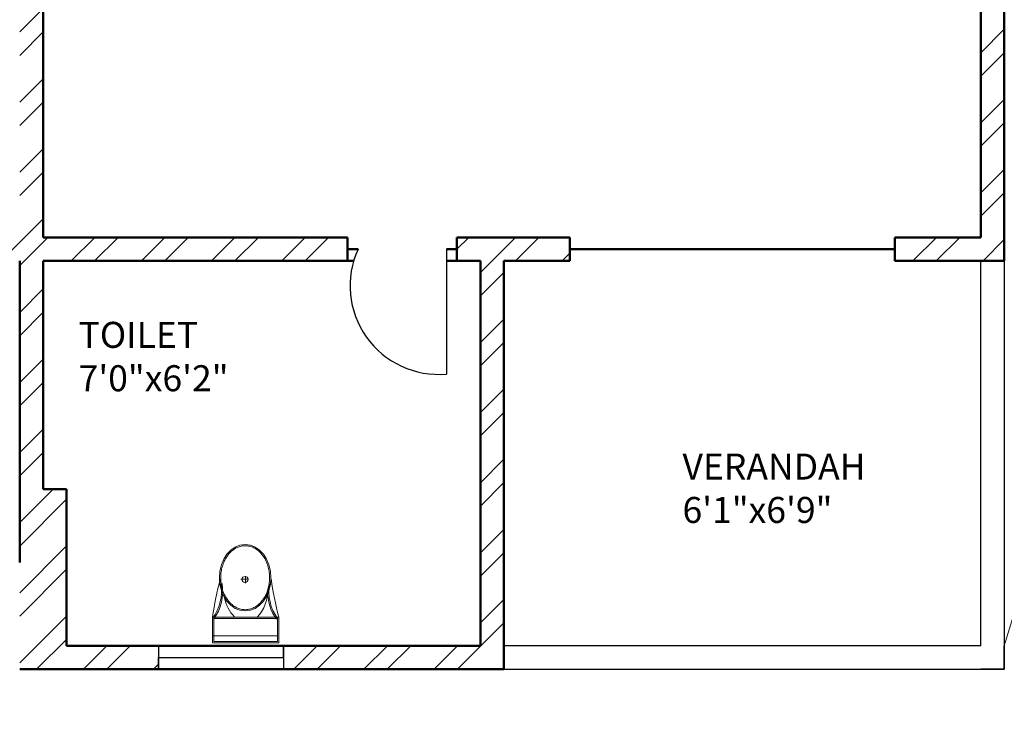
# Model space of a CAD drawing. Units: inches. Extents: x 1901 to 2863, y 888 to 2433.
# Tile 9 of 91: x 2154 to 2343, y 1216 to 1348. Entities that reach past the tile are written whole.
import ezdxf

# ---------------------------------------------------------------- set-up
doc = ezdxf.new("R2010")
doc.units = ezdxf.units.IN
for name, color, linetype, lineweight in [('A-ANNO-SYMB', 8, 'Continuous', 13), ('A-AREA-IDEN', 7, 'Continuous', 18), ('A-DOOR', 4, 'Continuous', 25), ('A-FLOR-FIXT', 9, 'Continuous', 18), ('A-FLOR-HRAL', 41, 'Continuous', 25), ('A-GLAZ', 3, 'Continuous', 25), ('A-WALL', 7, 'Continuous', 50), ('A-WALL-PATT', 8, 'Continuous', 13)]:
    doc.layers.add(name, color=color, linetype=linetype, lineweight=lineweight)
doc.styles.get("Standard").update_dxf_attribs({"font": 'arial.ttf'})

# ---------------------------------------------------------------- blocks, each defined once
blk = doc.blocks.new('A$C31115884')
for p, q in [((283.1, 497.7), (223.4, 497.7)), ((257.5, 466.4), (257.5, 523.2)), ((0, 200), (0, 0)), ((520, 200), (0, 200)), ((10, 190), (10, 10)), ((510, 190), (10, 190)), ((510, 10), (510, 190)), ((520, 0), (520, 200)), ((510, 54.5), (0, 54.5)), ((10, 10), (510, 10)), ((0, 0), (520, 0))]:
    blk.add_line(p, q)
blk.add_circle((255.6, 496.4), 23.6)
for centre, radius, start, end in [((2777.7, -204.6), 2807, 165.4549, 171.71327), ((-294.5, 403.3), 374.7, 324.20913, 9.34987), ((3237, 905), 2807, 188.28673, 194.5451), ((-294.5, 403.3), 364.7, 324.20913, 9.34987), ((139.5, 406.2), 293.5, 315.84364, 2.65635), ((805.8, 403.3), 374.7, 179.20365, 215.79087), ((805.8, 403.3), 364.7, 170.65013, 215.79087), ((383.6, 406.2), 293.5, 190.27735, 224.15636)]:
    blk.add_arc(centre, radius, start, end)
blk.add_ellipse((256.2, 509.9), major_axis=(0, -260.7), ratio=0.772727)
blk.add_open_spline([(256.2, 259.2), (263.1, 259.2), (270, 259.7), (287.8, 262.3), (298.7, 265.1), (319.9, 273.1), (330.2, 278.4), (350.1, 291.1), (359.7, 298.7), (377.7, 315.9), (386.2, 325.5), (401.7, 346.6), (408.8, 358.1), (421.3, 382.5), (426.8, 395.5), (435.9, 422.4), (439.5, 436.4), (444.8, 465.1), (446.5, 479.7), (447.9, 509.2), (447.6, 524), (445, 553.3), (442.7, 567.8), (436.3, 596), (432.1, 609.7), (421.9, 636), (416, 648.6), (402.5, 672.1), (395, 683), (378.6, 703), (369.8, 712.1), (351.1, 728), (341.3, 734.8), (320.9, 746.2), (310.4, 750.7), (288.9, 757.3), (278, 759.4), (256, 761), (245, 760.6), (223.1, 757.2), (212.3, 754.3), (191.1, 746.1), (180.8, 740.7), (160.9, 727.8), (151.4, 720.1), (133.5, 702.7), (125.1, 693), (109.6, 671.7), (102.6, 660.2), (90.2, 635.7), (84.9, 622.7), (76, 595.6), (72.4, 581.6), (67.2, 552.9), (65.6, 538.2), (64.4, 508.8), (64.8, 494), (67.5, 464.7), (69.9, 450.2), (76.6, 422), (80.8, 408.3), (91.1, 382.2), (97.2, 369.7), (110.8, 346.3), (118.4, 335.4), (134.8, 315.6), (143.7, 306.7), (162.4, 290.9), (172.3, 284.2), (192.8, 273), (203.3, 268.6), (224.8, 262.2), (235.8, 260.2), (249.9, 259.3), (253, 259.2), (256.2, 259.2)], degree=3, knots=[0, 0, 0, 0, 0.110105, 0.110105, 0.285049, 0.285049, 0.459994, 0.459994, 0.634938, 0.634938, 0.809882, 0.809882, 0.984827, 0.984827, 1.159771, 1.159771, 1.334715, 1.334715, 1.50966, 1.50966, 1.684604, 1.684604, 1.859549, 1.859549, 2.034493, 2.034493, 2.209437, 2.209437, 2.384382, 2.384382, 2.559326, 2.559326, 2.73427, 2.73427, 2.909215, 2.909215, 3.084159, 3.084159, 3.259103, 3.259103, 3.434048, 3.434048, 3.608992, 3.608992, 3.783936, 3.783936, 3.958881, 3.958881, 4.133825, 4.133825, 4.30877, 4.30877, 4.483714, 4.483714, 4.658658, 4.658658, 4.833603, 4.833603, 5.008547, 5.008547, 5.183491, 5.183491, 5.358436, 5.358436, 5.53338, 5.53338, 5.708324, 5.708324, 5.883269, 5.883269, 6.058213, 6.058213, 6.233158, 6.233158, 6.283185, 6.283185, 6.283185, 6.283185])
blk = doc.blocks.new('WIN-24')
for p, q in [((0, 4.5), (0, 0)), ((24, 2.25), (24, 4.5)), ((24, 4.5), (24, 0)), ((0, 0), (0, 2.25)), ((0, 2.25), (24, 2.25))]:
    blk.add_line(p, q)

msp = doc.modelspace()

# ---------------------------------------------------------------- hatches: boundary and pattern name
at = {"layer": 'A-WALL-PATT'}
h = msp.add_hatch(dxfattribs=at)
h.set_pattern_fill('ANSI32', color=256)
h.paths.add_polyline_path([(2192.5, 2274.13), (2141.26, 2274.13), (2141.26, 2269.63), (2192.5, 2269.63)])
h.paths.add_polyline_path([(2259.93, 2274.13), (2216.5, 2274.13), (2216.5, 2269.63), (2255.43, 2269.63), (2255.43, 2214.63), (2250.81, 2214.63), (2250.81, 2210.13), (2259.93, 2210.13), (2259.93, 2215.13), (2271.76, 2215.13), (2271.76, 2217.38), (2271.76, 2219.63), (2259.93, 2219.63)])
h.paths.add_polyline_path([(2171.43, 2269.63), (2166.93, 2269.63), (2166.93, 2219.63), (2121.24, 2219.63), (2121.24, 2215.13), (2166.93, 2215.13), (2166.93, 2083.13), (2161.81, 2083.13), (2161.81, 2078.63), (2171.43, 2078.63), (2177, 2078.63), (2177, 2080.88), (2177, 2083.13), (2171.43, 2083.13), (2171.43, 2210.13), (2230.91, 2210.13), (2230.91, 2212.38), (2230.91, 2214.63), (2171.43, 2214.63)])
h.paths.add_polyline_path([(2117.26, 2274.13), (2089.43, 2274.13), (2089.43, 2219.63), (2081.14, 2219.63), (2081.14, 2215.13), (2089.43, 2215.13), (2098, 2215.13), (2098, 2217.38), (2098, 2219.63), (2093.93, 2219.63), (2093.93, 2269.63), (2117.26, 2269.63), (2117.26, 2271.88)])
h.paths.add_polyline_path([(2343.43, 2219.63), (2329.29, 2219.63), (2329.29, 2215.13), (2338.93, 2215.13), (2338.93, 2184.74), (2343.43, 2184.74)])
h.paths.add_polyline_path([(2338.93, 2083.13), (2329.29, 2083.13), (2208.97, 2083.13), (2208.97, 2078.63), (2338.93, 2078.63)])
h.paths.add_polyline_path([(2343.43, 2136.74), (2338.93, 2136.74), (2338.93, 1872.63), (2343.43, 1872.63)])
h.paths.add_polyline_path([(2343.43, 1863.63), (2397.68, 1863.63), (2397.68, 1821.63), (2384.14, 1821.63), (2384.14, 1812.63), (2418.33, 1812.63), (2418.33, 1817.13), (2418.33, 1821.63), (2406.68, 1821.63), (2406.68, 1863.63), (2459.5, 1863.63), (2459.5, 1821.63), (2447.14, 1821.63), (2447.14, 1812.63), (2459.5, 1812.63), (2468.5, 1812.63), (2468.5, 1872.63), (2394.43, 1872.63), (2334.43, 1872.63), (2334.43, 1812.63), (2343.43, 1812.63), (2353.25, 1812.63), (2353.25, 1821.63), (2343.43, 1821.63)])
h.paths.add_polyline_path([(2510.01, 1872.63), (2468.5, 1872.63), (2468.5, 1868.13), (2510.01, 1868.13)])
h.paths.add_polyline_path([(2514.01, 1817.13), (2468.5, 1817.13), (2468.5, 1812.63), (2482.11, 1812.63), (2482.11, 1800.61), (2486.61, 1800.61), (2486.61, 1812.63), (2514.01, 1812.63)])
h.paths.add_polyline_path([(2299.25, 1814.88), (2299.25, 1817.13), (2295.93, 1817.13), (2295.93, 1854.17), (2293.68, 1854.17), (2291.43, 1854.17), (2291.43, 1817.13), (2266.11, 1817.13), (2266.11, 1812.63), (2299.25, 1812.63)])
h.paths.add_polyline_path([(2218.11, 1817.13), (2206.46, 1817.13), (2171.43, 1817.13), (2171.43, 1949.13), (2190.1, 1949.13), (2190.1, 1953.63), (2163.47, 1953.63), (2163.47, 1949.13), (2166.93, 1949.13), (2166.93, 1817.13), (2114.3, 1817.13), (2114.3, 1812.63), (2218.11, 1812.63)])
h.paths.add_polyline_path([(2029.43, 1970.92), (2024.93, 1970.92), (2024.93, 1912.72), (2029.43, 1912.72)])
h.paths.add_polyline_path([(2132.3, 1953.63), (2113.93, 1953.63), (2113.93, 1975.89), (2111.68, 1975.89), (2109.43, 1975.89), (2109.43, 1953.63), (2029.43, 1953.63), (2029.43, 1949.13), (2132.3, 1949.13)])
h.paths.add_polyline_path([(2029.43, 1853.61), (2029.31, 1853.61), (2029.31, 1853.61), (2029.43, 1853.61), (2029.43, 1864.72), (2024.93, 1864.72), (2024.93, 1812.63), (2066.3, 1812.63), (2066.3, 1814.88), (2066.3, 1817.13), (2029.43, 1817.13)])
h.paths.add_polyline_path([(2122.93, 2010.09), (2120.68, 2010.09), (2118.43, 2010.09), (2118.43, 2006.13), (2029.43, 2006.13), (2029.43, 2001.63), (2109.43, 2001.63), (2109.43, 1998.04), (2113.93, 1998.04), (2113.93, 2001.63), (2122.93, 2001.63)])
h.paths.add_polyline_path([(2029.43, 2031.38), (2024.93, 2031.38), (2024.93, 1994.92), (2027.18, 1994.92), (2029.43, 1994.92)])
h.paths.add_polyline_path([(2029.43, 2136.74), (2024.93, 2136.74), (2024.93, 2067.38), (2027.18, 2067.38), (2029.43, 2067.38)])
h.paths.add_polyline_path([(2125.62, 2083.13), (2029.43, 2083.13), (2029.43, 2078.63), (2118.43, 2078.63), (2118.43, 2030.71), (2122.93, 2030.71), (2122.93, 2078.63), (2125.62, 2078.63)])
h.paths.add_polyline_path([(2029.43, 2215.13), (2040.47, 2215.13), (2040.47, 2217.38), (2040.47, 2219.63), (2024.93, 2219.63), (2024.93, 2184.74), (2029.43, 2184.74), (2029.43, 2187.78)])
h.paths.add_polyline_path([(2686.43, 2274.13), (2659.28, 2274.13), (2659.28, 2269.63), (2681.93, 2269.63), (2681.93, 2219.63), (2676.82, 2219.63), (2676.82, 2215.13), (2681.93, 2215.13), (2697.01, 2215.13), (2697.01, 2217.38), (2697.01, 2219.63), (2686.43, 2219.63)])
h.paths.add_polyline_path([(2609.93, 2269.63), (2635.28, 2269.63), (2635.28, 2274.13), (2571.43, 2274.13), (2571.43, 2269.63), (2605.43, 2269.63), (2605.43, 2214.63), (2549.1, 2214.63), (2549.1, 2210.13), (2605.43, 2210.13), (2605.43, 2083.13), (2601.01, 2083.13), (2601.01, 2080.88), (2601.01, 2078.63), (2609.93, 2078.63), (2616.16, 2078.63), (2616.16, 2080.88), (2616.16, 2083.13), (2609.93, 2083.13), (2609.93, 2215.13), (2651.46, 2215.13), (2651.46, 2217.38), (2651.46, 2219.63), (2609.93, 2219.63)])
h.paths.add_polyline_path([(2521.43, 2269.63), (2547.43, 2269.63), (2547.43, 2271.88), (2547.43, 2274.13), (2516.93, 2274.13), (2516.93, 2219.63), (2506.41, 2219.63), (2506.41, 2215.13), (2516.93, 2215.13), (2516.93, 2210.13), (2525.4, 2210.13), (2525.4, 2212.38), (2525.4, 2214.63), (2521.43, 2214.63)])
h.paths.add_polyline_path([(2456.01, 2219.63), (2439.43, 2219.63), (2439.43, 2187.89), (2443.93, 2187.89), (2443.93, 2215.13), (2456.01, 2215.13)])
h.paths.add_polyline_path([(2752.93, 2219.63), (2739.48, 2219.63), (2739.48, 2215.13), (2748.43, 2215.13), (2748.43, 2187.89), (2752.93, 2187.89)])
h.paths.add_polyline_path([(2752.93, 2139.89), (2748.43, 2139.89), (2748.43, 2083.13), (2648.42, 2083.13), (2648.42, 2078.63), (2654.93, 2078.63), (2654.93, 2039.44), (2659.43, 2039.44), (2659.43, 2078.63), (2748.43, 2078.63), (2748.43, 2063.43), (2752.93, 2063.43)])
h.paths.add_polyline_path([(2752.93, 2010.63), (2659.43, 2010.63), (2659.43, 2015.65), (2654.93, 2015.65), (2654.93, 2010.63), (2605.43, 2010.63), (2605.43, 1920.97), (2609.93, 1920.97), (2609.93, 2006.13), (2748.43, 2006.13), (2748.43, 1982.47), (2752.93, 1982.47)])
h.paths.add_polyline_path([(2752.93, 2027.43), (2748.43, 2027.43), (2748.43, 2010.63), (2752.93, 2010.63)])
h.paths.add_polyline_path([(2748.43, 1886.13), (2609.93, 1886.13), (2609.93, 1889.72), (2605.43, 1889.72), (2605.43, 1861.26), (2609.93, 1861.26), (2609.93, 1881.63), (2748.43, 1881.63)])
h.paths.add_polyline_path([(2456.86, 2228.83), (2498.4, 2228.83), (2498.4, 2247.49), (2456.86, 2247.49)], flags=9)
h.paths.add_polyline_path([(2038.6, 2237.42), (2080.17, 2237.42), (2080.17, 2256.08), (2038.6, 2256.08)], flags=9)
h.paths.add_polyline_path([(2292.01, 1062.39), (2539.93, 1062.39), (2539.93, 1099.49), (2292.01, 1099.49)], flags=9)
h.paths.add_polyline_path([(2424.91, 1832.25), (2448.51, 1832.25), (2448.51, 1846.68), (2424.91, 1846.68)], flags=25)
h.paths.add_polyline_path([(2359.08, 1832.25), (2382.68, 1832.25), (2382.68, 1846.68), (2359.08, 1846.68)], flags=25)
h.paths.add_polyline_path([(2352.9, 1684.8), (2367.54, 1684.8), (2367.54, 1697.17), (2352.9, 1697.17)], flags=9)
h.paths.add_polyline_path([(2079.29, 1755.83), (2169.02, 1755.83), (2169.02, 1774.37), (2079.29, 1774.37)], flags=9)
h.paths.add_polyline_path([(2404.09, 1373.86), (2404.09, 1463.59), (2385.54, 1463.59), (2385.54, 1373.86)], flags=9)
h.paths.add_polyline_path([(2268.09, 2236.37), (2309.64, 2236.37), (2309.64, 2255.03), (2268.09, 2255.03)], flags=9)
h.paths.add_polyline_path([(2575.96, 1700.95), (2665.7, 1700.95), (2665.7, 1719.5), (2575.96, 1719.5)], flags=9)
h.paths.add_polyline_path([(2302.96, 1878.47), (2329.52, 1878.47), (2329.52, 1888.78), (2302.96, 1888.78)], flags=9)
h.paths.add_polyline_path([(2097.42, 2240.58), (2126.57, 2240.58), (2126.57, 2259.23), (2097.42, 2259.23)], flags=9)
h.paths.add_polyline_path([(2208.72, 2246.12), (2237.88, 2246.12), (2237.88, 2264.78), (2208.72, 2264.78)], flags=9)
h.paths.add_polyline_path([(2038.15, 1925.96), (2076.99, 1925.96), (2076.99, 1944.62), (2038.15, 1944.62)], flags=9)
h.paths.add_polyline_path([(2239.14, 1926.67), (2288.46, 1926.67), (2288.46, 1945.33), (2239.14, 1945.33)], flags=9)
h.paths.add_polyline_path([(2175.43, 2007.33), (2212.36, 2007.33), (2212.36, 2025.99), (2175.43, 2025.99)], flags=9)
h.paths.add_polyline_path([(2225.03, 2091.79), (2263.87, 2091.79), (2263.87, 2110.45), (2225.03, 2110.45)], flags=9)
h.paths.add_polyline_path([(2035.4, 2098.48), (2074.24, 2098.48), (2074.24, 2117.14), (2035.4, 2117.14)], flags=9)
h.paths.add_polyline_path([(2050.1, 2029.21), (2083.26, 2029.21), (2083.26, 2047.87), (2050.1, 2047.87)], flags=9)
h.paths.add_polyline_path([(2069.68, 1956.72), (2098.83, 1956.72), (2098.83, 1975.38), (2069.68, 1975.38)], flags=25)
h.paths.add_polyline_path([(2328.62, 1753.34), (2361.66, 1753.34), (2361.66, 1771.99), (2328.62, 1771.99)], flags=9)
h.paths.add_polyline_path([(2395.16, 2060.89), (2395.16, 2140.65), (2378.68, 2140.65), (2378.68, 2060.89)], flags=9)
h.paths.add_polyline_path([(2463.73, 2059.02), (2492.89, 2059.02), (2492.89, 2077.68), (2463.73, 2077.68)], flags=9)
h.paths.add_polyline_path([(2458.03, 2181.54), (2496.87, 2181.54), (2496.87, 2200.19), (2458.03, 2200.19)], flags=9)
h.paths.add_polyline_path([(2527.58, 2243.07), (2556.73, 2243.07), (2556.73, 2261.73), (2527.58, 2261.73)], flags=9)
h.paths.add_polyline_path([(2694.46, 2232.77), (2736.03, 2232.77), (2736.03, 2251.42), (2694.46, 2251.42)], flags=9)
h.paths.add_polyline_path([(2637.82, 2249.22), (2666.98, 2249.22), (2666.98, 2267.88), (2637.82, 2267.88)], flags=9)
h.paths.add_polyline_path([(2623.69, 2183.54), (2662.53, 2183.54), (2662.53, 2202.2), (2623.69, 2202.2)], flags=9)
h.paths.add_polyline_path([(2691.97, 2021.5), (2725.12, 2021.5), (2725.12, 2040.16), (2691.97, 2040.16)], flags=9)
h.paths.add_polyline_path([(2621.04, 1975.91), (2662.34, 1975.91), (2662.34, 1994.57), (2621.04, 1994.57)], flags=25)
h.paths.add_polyline_path([(2479.03, 1927.62), (2519.84, 1927.62), (2519.84, 1946.28), (2479.03, 1946.28)], flags=9)
h.paths.add_polyline_path([(2670.94, 1849.08), (2716.01, 1849.08), (2716.01, 1867.73), (2670.94, 1867.73)], flags=9)
h.paths.add_polyline_path([(2523.61, 1782.96), (2550.17, 1782.96), (2550.17, 1793.26), (2523.61, 1793.26)], flags=9)
h.paths.add_polyline_path([(2450.84, 1207.33), (2492.39, 1207.33), (2492.39, 1225.99), (2450.84, 1225.99)], flags=9)
h.paths.add_polyline_path([(2527.75, 1203.84), (2556.91, 1203.84), (2556.91, 1222.5), (2527.75, 1222.5)], flags=9)
h.paths.add_polyline_path([(2639.11, 1207.2), (2668.27, 1207.2), (2668.27, 1225.86), (2639.11, 1225.86)], flags=9)
h.paths.add_polyline_path([(2692.59, 1218.97), (2734.17, 1218.97), (2734.17, 1237.62), (2692.59, 1237.62)], flags=9)
h.paths.add_polyline_path([(2669.27, 1366.33), (2708.11, 1366.33), (2708.11, 1384.99), (2669.27, 1384.99)], flags=9)
h.paths.add_polyline_path([(2463.31, 1358.03), (2502.15, 1358.03), (2502.15, 1376.69), (2463.31, 1376.69)], flags=9)
h.paths.add_polyline_path([(2494.72, 1449.96), (2531.65, 1449.96), (2531.65, 1468.62), (2494.72, 1468.62)], flags=9)
h.paths.add_polyline_path([(2675.57, 1422.16), (2708.72, 1422.16), (2708.72, 1440.81), (2675.57, 1440.81)], flags=9)
h.paths.add_polyline_path([(2685.63, 1493.89), (2714.79, 1493.89), (2714.79, 1512.55), (2685.63, 1512.55)], flags=9)
h.paths.add_polyline_path([(2686.8, 1529.91), (2725.65, 1529.91), (2725.65, 1548.57), (2686.8, 1548.57)], flags=9)
h.paths.add_polyline_path([(2503.65, 1537.99), (2552.97, 1537.99), (2552.97, 1556.65), (2503.65, 1556.65)], flags=9)
h.paths.add_polyline_path([(2291.71, 1643.5), (2318.28, 1643.5), (2318.28, 1653.81), (2291.71, 1653.81)], flags=9)
h.paths.add_polyline_path([(2450.63, 1610.52), (2477.19, 1610.52), (2477.19, 1620.82), (2450.63, 1620.82)], flags=9)
h.paths.add_polyline_path([(2359.99, 1551.81), (2422.25, 1551.81), (2422.25, 1562.12), (2359.99, 1562.12)], flags=9)
h.paths.add_polyline_path([(2280.11, 1249.01), (2321.65, 1249.01), (2321.65, 1267.66), (2280.11, 1267.66)], flags=9)
h.paths.add_polyline_path([(2164.06, 1274.23), (2193.22, 1274.23), (2193.22, 1292.89), (2164.06, 1292.89)], flags=9)
h.paths.add_polyline_path([(2118.21, 1277.69), (2151.25, 1277.69), (2151.25, 1296.35), (2118.21, 1296.35)], flags=9)
h.paths.add_polyline_path([(2031.95, 1268.53), (2073.52, 1268.53), (2073.52, 1287.19), (2031.95, 1287.19)], flags=9)
h.paths.add_polyline_path([(2050.2, 1409.08), (2089.04, 1409.08), (2089.04, 1427.74), (2050.2, 1427.74)], flags=9)
h.paths.add_polyline_path([(2243.74, 1421.03), (2282.58, 1421.03), (2282.58, 1439.69), (2243.74, 1439.69)], flags=9)
h.paths.add_polyline_path([(2190.75, 1509.77), (2231.56, 1509.77), (2231.56, 1528.43), (2190.75, 1528.43)], flags=9)
h.paths.add_polyline_path([(2058.39, 1475.42), (2091.55, 1475.42), (2091.55, 1494.07), (2058.39, 1494.07)], flags=9)
h.paths.add_polyline_path([(2062.45, 1553.09), (2091.6, 1553.09), (2091.6, 1571.75), (2062.45, 1571.75)], flags=9)
h.paths.add_polyline_path([(2219.52, 1590.37), (2266.15, 1590.37), (2266.15, 1609.02), (2219.52, 1609.02)], flags=9)
h.paths.add_polyline_path([(2041.07, 1584.19), (2079.91, 1584.19), (2079.91, 1602.85), (2041.07, 1602.85)], flags=9)
h = msp.add_hatch(dxfattribs=at)
h.set_pattern_fill('ANSI32', color=256)
h.paths.add_polyline_path([(2443.93, 2139.89), (2439.43, 2139.89), (2439.43, 2069.35), (2441.68, 2069.35), (2443.93, 2069.35), (2443.93, 2078.63), (2521.93, 2078.63), (2521.93, 2075.07), (2524.18, 2075.07), (2526.43, 2075.07), (2526.43, 2078.63), (2571.75, 2078.63), (2571.75, 2080.88), (2571.75, 2083.13), (2443.93, 2083.13)])
h.paths.add_polyline_path([(2526.43, 2054.63), (2524.18, 2054.63), (2521.93, 2054.63), (2521.93, 2030.63), (2443.93, 2030.63), (2443.93, 2045.35), (2439.43, 2045.35), (2439.43, 1983.87), (2443.93, 1983.87), (2443.93, 2026.13), (2521.93, 2026.13), (2526.43, 2026.13)])
h.paths.add_polyline_path([(2443.93, 1923.87), (2439.43, 1923.87), (2439.43, 1872.63), (2443.93, 1872.63)])
h.paths.add_polyline_path([(2636.23, 1766.13), (2609.93, 1766.13), (2609.93, 1779.79), (2605.43, 1779.79), (2605.43, 1766.13), (2486.61, 1766.13), (2486.61, 1770.67), (2482.11, 1770.67), (2482.11, 1766.13), (2482.11, 1761.63), (2636.23, 1761.63), (2636.23, 1763.88)])
h.paths.add_polyline_path([(2519.54, 1663.38), (2519.54, 1665.63), (2494.93, 1665.63), (2481.83, 1665.63), (2481.83, 1663.38), (2481.83, 1661.13), (2490.43, 1661.13), (2490.43, 1640.16), (2494.93, 1640.16), (2494.93, 1661.13), (2519.54, 1661.13)])
h.paths.add_polyline_path([(2443.93, 1712.13), (2443.93, 1716.63), (2414.46, 1716.63), (2414.46, 1712.13), (2439.43, 1712.13), (2439.43, 1545.51), (2443.93, 1545.51), (2443.93, 1661.13), (2448.47, 1661.13), (2448.47, 1665.63), (2443.93, 1665.63)])
h.paths.add_polyline_path([(2343.43, 1712.13), (2365.52, 1712.13), (2365.52, 1714.38), (2365.52, 1716.63), (2333.87, 1716.63), (2333.87, 1714.38), (2333.87, 1712.13), (2338.93, 1712.13), (2338.93, 1575.63), (2338.93, 1545.51), (2343.43, 1545.51), (2343.43, 1547.51), (2343.43, 1580.13)])
h.paths.add_polyline_path([(2752.93, 1665.63), (2579.54, 1665.63), (2579.54, 1661.13), (2615.93, 1661.13), (2615.93, 1529.13), (2598.93, 1529.13), (2598.93, 1524.63), (2623.13, 1524.63), (2623.13, 1526.88), (2623.13, 1529.13), (2620.43, 1529.13), (2620.43, 1661.13), (2748.43, 1661.13), (2748.43, 1633.5), (2752.93, 1633.5)])
h.paths.add_polyline_path([(2752.93, 1419.93), (2748.43, 1419.93), (2748.43, 1400.13), (2659.43, 1400.13), (2659.43, 1444.33), (2657.18, 1444.33), (2654.93, 1444.33), (2654.93, 1400.13), (2643.65, 1400.13), (2643.65, 1395.63), (2748.43, 1395.63), (2748.43, 1364.04), (2752.93, 1364.04)])
h.paths.add_polyline_path([(2752.93, 1492.88), (2748.43, 1492.88), (2748.43, 1476.63), (2667.43, 1476.63), (2667.43, 1479.71), (2665.18, 1479.71), (2662.93, 1479.71), (2662.93, 1476.63), (2654.93, 1476.63), (2654.93, 1469.54), (2659.43, 1469.54), (2659.43, 1472.13), (2748.43, 1472.13), (2748.43, 1455.93), (2752.93, 1455.93)])
h.paths.add_polyline_path([(2752.93, 1304.04), (2748.43, 1304.04), (2748.43, 1263.63), (2738.66, 1263.63), (2738.66, 1259.13), (2752.93, 1259.13)])
h.paths.add_polyline_path([(2685.93, 1259.13), (2695.49, 1259.13), (2695.49, 1261.38), (2695.49, 1263.63), (2677.84, 1263.63), (2677.84, 1261.38), (2677.84, 1259.13), (2681.43, 1259.13), (2681.43, 1203.63), (2653.28, 1203.63), (2653.28, 1199.13), (2685.93, 1199.13), (2685.93, 1203.63)])
h.paths.add_polyline_path([(2609.43, 1395.63), (2611.85, 1395.63), (2611.85, 1400.13), (2598.89, 1400.13), (2598.89, 1397.88), (2598.89, 1395.63), (2604.93, 1395.63), (2604.93, 1268.13), (2554.73, 1268.13), (2554.73, 1265.88), (2554.73, 1263.63), (2604.93, 1263.63), (2604.93, 1203.63), (2571.31, 1203.63), (2571.31, 1199.13), (2604.93, 1199.13), (2629.28, 1199.13), (2629.28, 1201.38), (2629.28, 1203.63), (2609.43, 1203.63), (2609.43, 1258.63), (2609.43, 1259.13), (2654.8, 1259.13), (2654.8, 1263.63), (2609.43, 1263.63)])
h.paths.add_polyline_path([(2443.93, 1304.04), (2439.43, 1304.04), (2439.43, 1259.13), (2443.93, 1259.13), (2456.16, 1259.13), (2456.16, 1261.38), (2456.16, 1263.63), (2443.93, 1263.63)])
h.paths.add_polyline_path([(2525.43, 1263.63), (2531.78, 1263.63), (2531.78, 1268.13), (2520.93, 1268.13), (2520.93, 1263.63), (2511.41, 1263.63), (2511.41, 1259.13), (2520.93, 1259.13), (2520.93, 1199.13), (2547.31, 1199.13), (2547.31, 1201.38), (2547.31, 1203.63), (2525.43, 1203.63)])
h.paths.add_polyline_path([(2443.93, 1434.84), (2439.43, 1434.84), (2439.43, 1364.04), (2441.68, 1364.04), (2443.93, 1364.04)])
h.paths.add_polyline_path([(2567.13, 1400.13), (2443.93, 1400.13), (2443.93, 1395.63), (2567.13, 1395.63)])
h.paths.add_polyline_path([(2443.93, 1545.51), (2439.43, 1545.51), (2439.43, 1494.84), (2443.93, 1494.84)])
h.paths.add_polyline_path([(2494.93, 1553.35), (2492.68, 1553.35), (2490.43, 1553.35), (2490.43, 1524.63), (2494.93, 1524.63), (2525.94, 1524.63), (2525.94, 1526.88), (2525.94, 1529.13), (2494.93, 1529.13)])
h.paths.add_polyline_path([(2752.93, 1573.5), (2748.43, 1573.5), (2748.43, 1529.13), (2657.76, 1529.13), (2657.76, 1524.63), (2662.93, 1524.63), (2662.93, 1498.63), (2667.43, 1498.63), (2667.43, 1524.63), (2748.43, 1524.63), (2748.43, 1516.88), (2752.93, 1516.88)])
h.paths.add_polyline_path([(2038.6, 2237.42), (2080.17, 2237.42), (2080.17, 2256.08), (2038.6, 2256.08)], flags=9)
h.paths.add_polyline_path([(2292.01, 1062.39), (2539.93, 1062.39), (2539.93, 1099.49), (2292.01, 1099.49)], flags=9)
h.paths.add_polyline_path([(2424.91, 1832.25), (2448.51, 1832.25), (2448.51, 1846.68), (2424.91, 1846.68)], flags=9)
h.paths.add_polyline_path([(2359.08, 1832.25), (2382.68, 1832.25), (2382.68, 1846.68), (2359.08, 1846.68)], flags=9)
h.paths.add_polyline_path([(2352.9, 1684.8), (2367.54, 1684.8), (2367.54, 1697.17), (2352.9, 1697.17)], flags=9)
h.paths.add_polyline_path([(2079.29, 1755.83), (2169.02, 1755.83), (2169.02, 1774.37), (2079.29, 1774.37)], flags=9)
h.paths.add_polyline_path([(2404.09, 1373.86), (2404.09, 1463.59), (2385.54, 1463.59), (2385.54, 1373.86)], flags=9)
h.paths.add_polyline_path([(2268.09, 2236.37), (2309.64, 2236.37), (2309.64, 2255.03), (2268.09, 2255.03)], flags=9)
h.paths.add_polyline_path([(2575.96, 1700.95), (2665.7, 1700.95), (2665.7, 1719.5), (2575.96, 1719.5)], flags=9)
h.paths.add_polyline_path([(2302.96, 1878.47), (2329.52, 1878.47), (2329.52, 1888.78), (2302.96, 1888.78)], flags=9)
h.paths.add_polyline_path([(2097.42, 2240.58), (2126.57, 2240.58), (2126.57, 2259.23), (2097.42, 2259.23)], flags=9)
h.paths.add_polyline_path([(2208.72, 2246.12), (2237.88, 2246.12), (2237.88, 2264.78), (2208.72, 2264.78)], flags=9)
h.paths.add_polyline_path([(2038.15, 1925.96), (2076.99, 1925.96), (2076.99, 1944.62), (2038.15, 1944.62)], flags=9)
h.paths.add_polyline_path([(2239.14, 1926.67), (2288.46, 1926.67), (2288.46, 1945.33), (2239.14, 1945.33)], flags=9)
h.paths.add_polyline_path([(2175.43, 2007.33), (2212.36, 2007.33), (2212.36, 2025.99), (2175.43, 2025.99)], flags=9)
h.paths.add_polyline_path([(2225.03, 2091.79), (2263.87, 2091.79), (2263.87, 2110.45), (2225.03, 2110.45)], flags=9)
h.paths.add_polyline_path([(2035.4, 2098.48), (2074.24, 2098.48), (2074.24, 2117.14), (2035.4, 2117.14)], flags=9)
h.paths.add_polyline_path([(2050.1, 2029.21), (2083.26, 2029.21), (2083.26, 2047.87), (2050.1, 2047.87)], flags=9)
h.paths.add_polyline_path([(2069.68, 1956.72), (2098.83, 1956.72), (2098.83, 1975.38), (2069.68, 1975.38)], flags=9)
h.paths.add_polyline_path([(2328.62, 1753.34), (2361.66, 1753.34), (2361.66, 1771.99), (2328.62, 1771.99)], flags=9)
h.paths.add_polyline_path([(2395.16, 2060.89), (2395.16, 2140.65), (2378.68, 2140.65), (2378.68, 2060.89)], flags=9)
h.paths.add_polyline_path([(2463.73, 2059.02), (2492.89, 2059.02), (2492.89, 2077.68), (2463.73, 2077.68)], flags=9)
h.paths.add_polyline_path([(2458.03, 2181.54), (2496.87, 2181.54), (2496.87, 2200.19), (2458.03, 2200.19)], flags=9)
h.paths.add_polyline_path([(2456.86, 2228.83), (2498.4, 2228.83), (2498.4, 2247.49), (2456.86, 2247.49)], flags=9)
h.paths.add_polyline_path([(2527.58, 2243.07), (2556.73, 2243.07), (2556.73, 2261.73), (2527.58, 2261.73)], flags=9)
h.paths.add_polyline_path([(2694.46, 2232.77), (2736.03, 2232.77), (2736.03, 2251.42), (2694.46, 2251.42)], flags=9)
h.paths.add_polyline_path([(2637.82, 2249.22), (2666.98, 2249.22), (2666.98, 2267.88), (2637.82, 2267.88)], flags=9)
h.paths.add_polyline_path([(2623.69, 2183.54), (2662.53, 2183.54), (2662.53, 2202.2), (2623.69, 2202.2)], flags=9)
h.paths.add_polyline_path([(2691.97, 2021.5), (2725.12, 2021.5), (2725.12, 2040.16), (2691.97, 2040.16)], flags=9)
h.paths.add_polyline_path([(2621.04, 1975.91), (2662.34, 1975.91), (2662.34, 1994.57), (2621.04, 1994.57)], flags=9)
h.paths.add_polyline_path([(2479.03, 1927.62), (2519.84, 1927.62), (2519.84, 1946.28), (2479.03, 1946.28)], flags=9)
h.paths.add_polyline_path([(2670.94, 1849.08), (2716.01, 1849.08), (2716.01, 1867.73), (2670.94, 1867.73)], flags=9)
h.paths.add_polyline_path([(2523.61, 1782.96), (2550.17, 1782.96), (2550.17, 1793.26), (2523.61, 1793.26)], flags=9)
h.paths.add_polyline_path([(2450.84, 1207.33), (2492.39, 1207.33), (2492.39, 1225.99), (2450.84, 1225.99)], flags=9)
h.paths.add_polyline_path([(2527.75, 1203.84), (2556.91, 1203.84), (2556.91, 1222.5), (2527.75, 1222.5)], flags=9)
h.paths.add_polyline_path([(2639.11, 1207.2), (2668.27, 1207.2), (2668.27, 1225.86), (2639.11, 1225.86)], flags=9)
h.paths.add_polyline_path([(2692.59, 1218.97), (2734.17, 1218.97), (2734.17, 1237.62), (2692.59, 1237.62)], flags=9)
h.paths.add_polyline_path([(2669.27, 1366.33), (2708.11, 1366.33), (2708.11, 1384.99), (2669.27, 1384.99)], flags=25)
h.paths.add_polyline_path([(2463.31, 1358.03), (2502.15, 1358.03), (2502.15, 1376.69), (2463.31, 1376.69)], flags=9)
h.paths.add_polyline_path([(2494.72, 1449.96), (2531.65, 1449.96), (2531.65, 1468.62), (2494.72, 1468.62)], flags=9)
h.paths.add_polyline_path([(2675.57, 1422.16), (2708.72, 1422.16), (2708.72, 1440.81), (2675.57, 1440.81)], flags=25)
h.paths.add_polyline_path([(2685.63, 1493.89), (2714.79, 1493.89), (2714.79, 1512.55), (2685.63, 1512.55)], flags=9)
h.paths.add_polyline_path([(2686.8, 1529.91), (2725.65, 1529.91), (2725.65, 1548.57), (2686.8, 1548.57)], flags=25)
h.paths.add_polyline_path([(2503.65, 1537.99), (2552.97, 1537.99), (2552.97, 1556.65), (2503.65, 1556.65)], flags=9)
h.paths.add_polyline_path([(2291.71, 1643.5), (2318.28, 1643.5), (2318.28, 1653.81), (2291.71, 1653.81)], flags=9)
h.paths.add_polyline_path([(2450.63, 1610.52), (2477.19, 1610.52), (2477.19, 1620.82), (2450.63, 1620.82)], flags=9)
h.paths.add_polyline_path([(2359.99, 1551.81), (2422.25, 1551.81), (2422.25, 1562.12), (2359.99, 1562.12)], flags=9)
h.paths.add_polyline_path([(2280.11, 1249.01), (2321.65, 1249.01), (2321.65, 1267.66), (2280.11, 1267.66)], flags=9)
h.paths.add_polyline_path([(2164.06, 1274.23), (2193.22, 1274.23), (2193.22, 1292.89), (2164.06, 1292.89)], flags=9)
h.paths.add_polyline_path([(2118.21, 1277.69), (2151.25, 1277.69), (2151.25, 1296.35), (2118.21, 1296.35)], flags=9)
h.paths.add_polyline_path([(2031.95, 1268.53), (2073.52, 1268.53), (2073.52, 1287.19), (2031.95, 1287.19)], flags=9)
h.paths.add_polyline_path([(2050.2, 1409.08), (2089.04, 1409.08), (2089.04, 1427.74), (2050.2, 1427.74)], flags=9)
h.paths.add_polyline_path([(2243.74, 1421.03), (2282.58, 1421.03), (2282.58, 1439.69), (2243.74, 1439.69)], flags=9)
h.paths.add_polyline_path([(2190.75, 1509.77), (2231.56, 1509.77), (2231.56, 1528.43), (2190.75, 1528.43)], flags=9)
h.paths.add_polyline_path([(2058.39, 1475.42), (2091.55, 1475.42), (2091.55, 1494.07), (2058.39, 1494.07)], flags=9)
h.paths.add_polyline_path([(2062.45, 1553.09), (2091.6, 1553.09), (2091.6, 1571.75), (2062.45, 1571.75)], flags=9)
h.paths.add_polyline_path([(2219.52, 1590.37), (2266.15, 1590.37), (2266.15, 1609.02), (2219.52, 1609.02)], flags=9)
h.paths.add_polyline_path([(2041.07, 1584.19), (2079.91, 1584.19), (2079.91, 1602.85), (2041.07, 1602.85)], flags=9)
h = msp.add_hatch(dxfattribs=at)
h.set_pattern_fill('ANSI32', color=256)
h.paths.add_polyline_path([(2182.93, 1716.63), (2024.93, 1716.63), (2024.93, 1681.7), (2029.33, 1681.7), (2029.33, 1712.13), (2154.33, 1712.13), (2154.33, 1580.13), (2148.52, 1580.13), (2148.52, 1577.88), (2148.52, 1575.63), (2194.93, 1575.63), (2194.93, 1580.13), (2158.83, 1580.13), (2158.83, 1712.13), (2182.93, 1712.13)])
h.paths.add_polyline_path([(2301.07, 1716.63), (2242.93, 1716.63), (2242.93, 1712.13), (2283.83, 1712.13), (2283.83, 1685.54), (2288.33, 1685.54), (2288.33, 1712.13), (2301.07, 1712.13)])
h.paths.add_polyline_path([(2288.33, 1600.41), (2286.08, 1600.41), (2283.83, 1600.41), (2283.83, 1580.13), (2270.6, 1580.13), (2270.6, 1575.63), (2288.33, 1575.63)])
h.paths.add_polyline_path([(2295.93, 1953.63), (2271.45, 1953.63), (2271.45, 1949.13), (2291.43, 1949.13), (2291.43, 1941.24), (2295.93, 1941.24)])
h.paths.add_polyline_path([(2098.38, 1244.13), (2082.33, 1244.13), (2082.33, 1302.13), (2086.52, 1302.13), (2086.52, 1306.63), (2067.46, 1306.63), (2067.46, 1302.13), (2077.83, 1302.13), (2077.83, 1239.63), (2098.38, 1239.63), (2098.38, 1241.88)])
h.paths.add_polyline_path([(2217.31, 1306.63), (2158.83, 1306.63), (2158.83, 1451.63), (2162.72, 1451.63), (2162.72, 1453.88), (2162.72, 1456.13), (2154.33, 1456.13), (2154.33, 1443.13), (2151.91, 1443.13), (2151.91, 1438.63), (2154.33, 1438.63), (2154.33, 1306.63), (2109.31, 1306.63), (2109.31, 1304.38), (2109.31, 1302.13), (2154.33, 1302.13), (2154.33, 1244.13), (2122.38, 1244.13), (2122.38, 1239.63), (2154.33, 1239.63), (2154.33, 1223.63), (2163.33, 1223.63), (2181.01, 1223.63), (2181.01, 1225.88), (2181.01, 1228.13), (2163.33, 1228.13), (2163.33, 1258.22), (2158.83, 1258.22), (2158.83, 1302.13), (2217.31, 1302.13)])
h.paths.add_polyline_path([(2259.99, 1306.63), (2238.3, 1306.63), (2238.3, 1304.38), (2238.3, 1302.13), (2242.83, 1302.13), (2242.83, 1228.13), (2205.01, 1228.13), (2205.01, 1223.63), (2247.33, 1223.63), (2247.33, 1302.13), (2259.99, 1302.13), (2259.99, 1304.38)])
h.paths.add_polyline_path([(2343.43, 1361.7), (2338.93, 1361.7), (2338.93, 1306.63), (2322.38, 1306.63), (2322.38, 1302.13), (2343.43, 1302.13)])
h.paths.add_polyline_path([(2343.43, 1470.4), (2338.93, 1470.4), (2338.93, 1456.13), (2193.73, 1456.13), (2193.73, 1453.88), (2193.73, 1451.63), (2338.93, 1451.63), (2338.93, 1421.7), (2343.43, 1421.7)])
h.paths.add_polyline_path([(2343.43, 1545.51), (2338.93, 1545.51), (2338.93, 1530.4), (2343.43, 1530.4)])
h.paths.add_polyline_path([(2029.33, 1466.83), (2024.93, 1466.83), (2024.93, 1409.82), (2029.33, 1409.82)])
h.paths.add_polyline_path([(2122.84, 1440.88), (2122.84, 1443.13), (2121.83, 1443.13), (2121.83, 1498.18), (2119.58, 1498.18), (2117.33, 1498.18), (2117.33, 1443.13), (2029.33, 1443.13), (2029.33, 1438.63), (2122.84, 1438.63)])
h.paths.add_polyline_path([(2029.33, 1543.05), (2024.93, 1543.05), (2024.93, 1502.83), (2029.33, 1502.83)])
h.paths.add_polyline_path([(2029.33, 1621.7), (2024.93, 1621.7), (2024.93, 1567.05), (2027.13, 1567.05), (2029.33, 1567.05), (2029.33, 1575.63), (2109.33, 1575.63), (2109.33, 1554.71), (2113.83, 1554.71), (2113.83, 1575.63), (2115.8, 1575.63), (2115.8, 1577.88), (2115.8, 1580.13), (2029.33, 1580.13)])
h.paths.add_polyline_path([(2121.83, 1527.63), (2117.33, 1527.63), (2113.83, 1527.63), (2113.83, 1533.01), (2111.58, 1533.01), (2109.33, 1533.01), (2109.33, 1527.63), (2029.33, 1527.63), (2029.33, 1523.13), (2117.33, 1523.13), (2117.33, 1519.43), (2121.83, 1519.43)])
h.paths.add_polyline_path([(2029.33, 1349.82), (2024.93, 1349.82), (2024.93, 1302.13), (2036.28, 1302.13), (2036.28, 1306.63), (2029.33, 1306.63)])

# ---------------------------------------------------------------- linework, layer by layer
at = {"layer": 'A-ANNO-SYMB'}
msp.add_line((2343.43, 1228.13), (2439.43, 1545.51), dxfattribs=at)
at = {"layer": 'A-DOOR'}
msp.add_line((2236.3, 1304.38), (2236.3, 1280.38), dxfattribs=at)
msp.add_arc((2234.79, 1297.33), 17.02, 155.518, 275.0742, dxfattribs=at)
at = {"layer": 'A-FLOR-HRAL'}
for p, q in [((2338.93, 1228.13), (2338.93, 1302.13)), ((2343.43, 1302.13), (2343.43, 1223.63)), ((2338.93, 1228.13), (2247.33, 1228.13)), ((2343.43, 1223.63), (2343.43, 1228.13)), ((2247.33, 1223.63), (2343.43, 1223.63)), ((2343.43, 1223.63), (2338.93, 1223.63))]:
    msp.add_line(p, q, dxfattribs=at)
at = {"layer": 'A-WALL'}
for p, q in [((2343.43, 1302.13), (2343.43, 1580.13)), ((2158.83, 1451.63), (2158.83, 1306.63)), ((2338.93, 1451.63), (2338.93, 1306.63)), ((2217.31, 1306.63), (2158.83, 1306.63)), ((2217.31, 1302.13), (2217.31, 1306.63)), ((2217.31, 1306.63), (2217.31, 1304.38)), ((2238.3, 1302.13), (2238.3, 1306.63)), ((2238.3, 1306.63), (2238.3, 1304.38)), ((2259.99, 1306.63), (2238.3, 1306.63)), ((2259.99, 1306.63), (2259.99, 1302.13)), ((2338.93, 1306.63), (2322.38, 1306.63)), ((2322.38, 1304.38), (2322.38, 1306.63)), ((2322.38, 1306.63), (2322.38, 1302.13)), ((2217.31, 1304.38), (2219.31, 1304.38)), ((2238.3, 1304.38), (2236.3, 1304.38)), ((2259.99, 1302.13), (2259.99, 1304.38)), ((2259.99, 1304.38), (2322.38, 1304.38)), ((2154.33, 1302.13), (2154.33, 1244.13)), ((2158.83, 1302.13), (2158.83, 1258.22)), ((2218.47, 1302.13), (2158.83, 1302.13)), ((2242.83, 1302.13), (2236.3, 1302.13)), ((2242.83, 1302.13), (2242.83, 1228.13)), ((2247.33, 1302.13), (2247.33, 1223.63)), ((2259.99, 1302.13), (2247.33, 1302.13)), ((2343.43, 1302.13), (2322.38, 1302.13)), ((2163.33, 1258.22), (2158.83, 1258.22)), ((2163.33, 1228.13), (2163.33, 1258.22)), ((2242.83, 1228.13), (2163.33, 1228.13)), ((2247.33, 1223.63), (2154.33, 1223.63)), ((2154.33, 1223.63), (2163.33, 1223.63))]:
    msp.add_line(p, q, dxfattribs=at)

# ---------------------------------------------------------------- block references
at = {"layer": 'A-FLOR-FIXT', "xscale": 0.0245149588751191, "yscale": 0.0245149588751191, "zscale": 0.0245149588751191}
msp.add_blockref('A$C31115884', (2191.35, 1228.73), dxfattribs=at)
at = {"layer": 'A-GLAZ'}
msp.add_blockref('WIN-24', (2181.01, 1223.63), dxfattribs=at)

# ---------------------------------------------------------------- texts
at = {"layer": 'A-AREA-IDEN', "char_height": 5, "attachment_point": 1}
for s, width, insert in [('TOILET\\P7\'0"x6\'2"', 143.1094, (2165.64, 1290.4)), ('VERANDAH\\P6\'1"x6\'9"', 152.0889, (2281.62, 1265.09))]:
    msp.add_mtext_dynamic_manual_height_columns(s, width=width, gutter_width=12.5, heights=[0], dxfattribs=dict(at, insert=insert))

doc.saveas('drawing.dxf')
